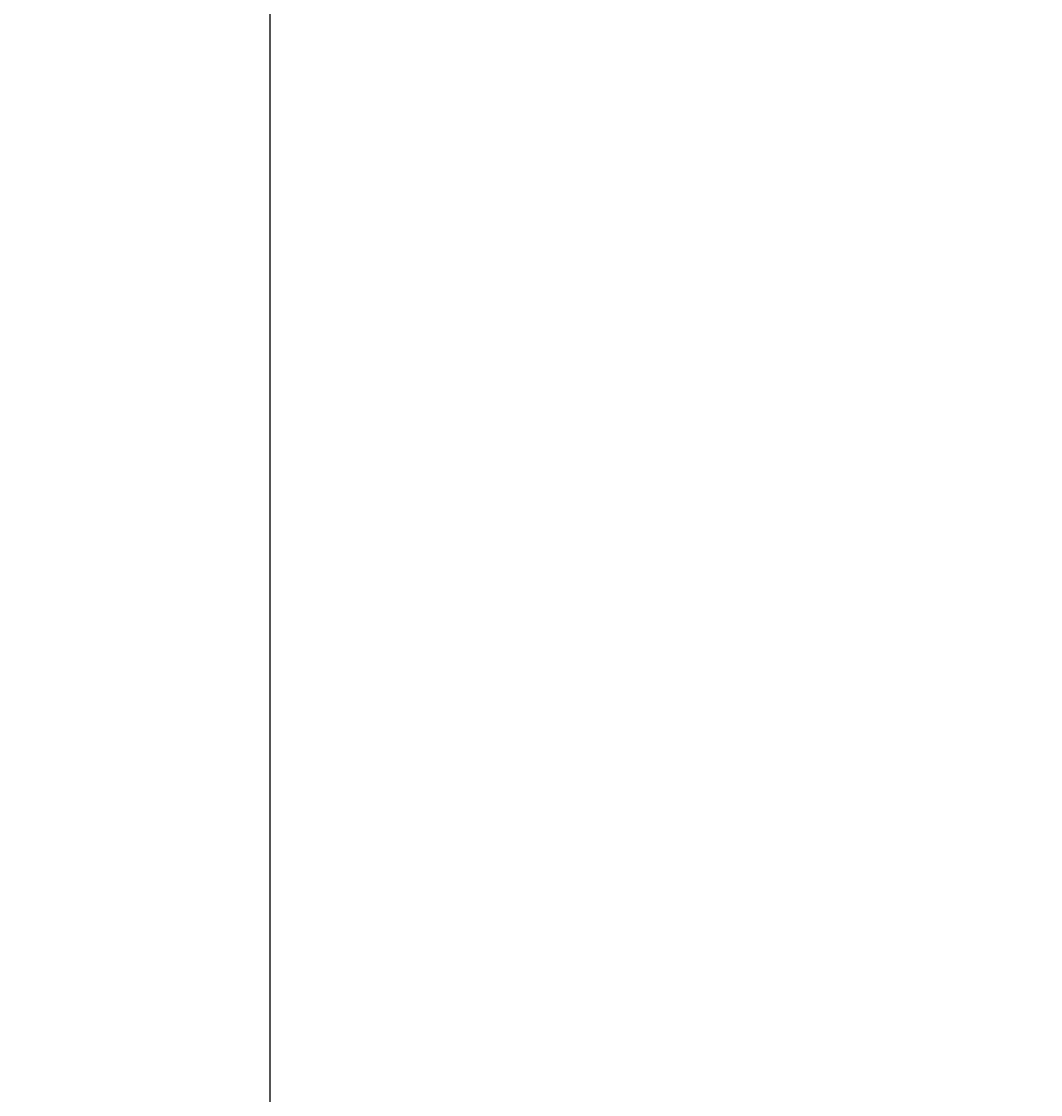
# Model space of a CAD drawing. Units: inches. Extents: x 1998 to 2588, y 1139 to 1977.
# Tile 27 of 134: x 2289 to 2316, y 1456 to 1484. Entities that reach past the tile are written whole.
import ezdxf

# ---------------------------------------------------------------- set-up
doc = ezdxf.new("R2010")
doc.units = ezdxf.units.IN
doc.layers.add('A-ANNO-DIMS', color=2, linetype='Continuous', lineweight=18)
doc.styles.get("Standard").update_dxf_attribs({"font": 'arial.ttf'})
doc.dimstyles.get("Standard").update_dxf_attribs({"dimtxt": 0.18, "dimasz": 0.18, "dimexe": 0.18, "dimexo": 0.0625, "dimgap": 0.09, "dimtad": 0, "dimtih": 1, "dimtoh": 1, "dimdec": 4, "dimzin": 0, "dimdsep": 46, "dimtxsty": 'Standard', "dimcen": 0.09, "dimadec": 0, "dimazin": 0, "dimtfac": 1, "dimtdec": 4, "dimtofl": 0, "dimtmove": 0, "dimatfit": 3, "dimfxl": 1, "dimtolj": 1, "dimtzin": 0, "dimarcsym": 0})

# ---------------------------------------------------------------- blocks, each defined once
blk = doc.blocks.new('*D23')
at = {"layer": 'A-ANNO-DIMS', "color": 0, "lineweight": -2, "transparency": 16777216}
for p, q in [((2549.179, 1476.17), (2549.179, 1138.602)), ((2059.473, 1413.17), (2059.473, 1138.602)), ((2059.653, 1138.782), (2303.928, 1138.782)), ((2548.999, 1138.782), (2304.723, 1138.782))]:
    blk.add_line(p, q, dxfattribs=at)
at = {"layer": 'A-ANNO-DIMS', "color": 0, "transparency": 16777216}
for points in [[(2059.653, 1138.812), (2059.653, 1138.752), (2059.473, 1138.782)], [(2548.999, 1138.812), (2548.999, 1138.752), (2549.179, 1138.782)]]:
    blk.add_solid(points, dxfattribs=at)
at = {"layer": 'Defpoints', "color": 0, "transparency": 16777216}
for p in [(2549.179, 1476.232), (2059.473, 1413.232), (2549.179, 1138.782)]:
    blk.add_point(p, dxfattribs=at)
at = {"layer": 'A-ANNO-DIMS', "color": 0, "transparency": 16777216, "insert": (2304.326, 1138.782), "char_height": 0.18, "attachment_point": 5}
blk.add_mtext('\\A1;489.7', dxfattribs=at)
blk = doc.blocks.new('*D44')
at = {"layer": 'A-ANNO-DIMS', "color": 0, "lineweight": -2, "transparency": 16777216}
for p, q in [((2295.414, 1588.67), (2295.414, 1138.602)), ((2337.287, 1588.67), (2337.287, 1138.602)), ((2295.594, 1138.782), (2315.953, 1138.782)), ((2337.107, 1138.782), (2316.748, 1138.782))]:
    blk.add_line(p, q, dxfattribs=at)
at = {"layer": 'A-ANNO-DIMS', "color": 0, "transparency": 16777216}
for points in [[(2295.594, 1138.812), (2295.594, 1138.752), (2295.414, 1138.782)], [(2337.107, 1138.812), (2337.107, 1138.752), (2337.287, 1138.782)]]:
    blk.add_solid(points, dxfattribs=at)
at = {"layer": 'Defpoints', "color": 0, "transparency": 16777216}
for p in [(2295.414, 1588.732), (2337.287, 1588.732), (2337.287, 1138.782)]:
    blk.add_point(p, dxfattribs=at)
at = {"layer": 'A-ANNO-DIMS', "color": 0, "transparency": 16777216, "insert": (2316.35, 1138.782), "char_height": 0.18, "attachment_point": 5}
blk.add_mtext('\\A1;41.87', dxfattribs=at)

msp = doc.modelspace()

# ---------------------------------------------------------------- dimensions: what is measured, and where the dimension line sits
at = {"layer": 'A-ANNO-DIMS'}
for base, p1, p2, override, picture, middle in [((2337.2869, 1138.7824), (2295.4138, 1588.7324), (2337.2869, 1588.7324), {"dimdec": 2, "dimlfac": 1, "dimrnd": 0, "dimzin": 0, "dimdsep": 46, "dimlunit": 2}, '*D44', (2316.3503, 1138.7824)), ((2549.1786, 1138.7824), (2059.4729, 1413.2324), (2549.1786, 1476.2324), {"dimdec": 1, "dimlfac": 1, "dimrnd": 0, "dimzin": 0, "dimdsep": 46, "dimlunit": 2}, '*D23', (2304.3257, 1138.7824))]:
    dim = msp.add_linear_dim(base=base, p1=p1, p2=p2, dimstyle='Standard', override=override, dxfattribs=at)
    dim.commit()
    dim.dimension.update_dxf_attribs({"geometry": picture, "text_midpoint": middle})

doc.saveas('drawing.dxf')
